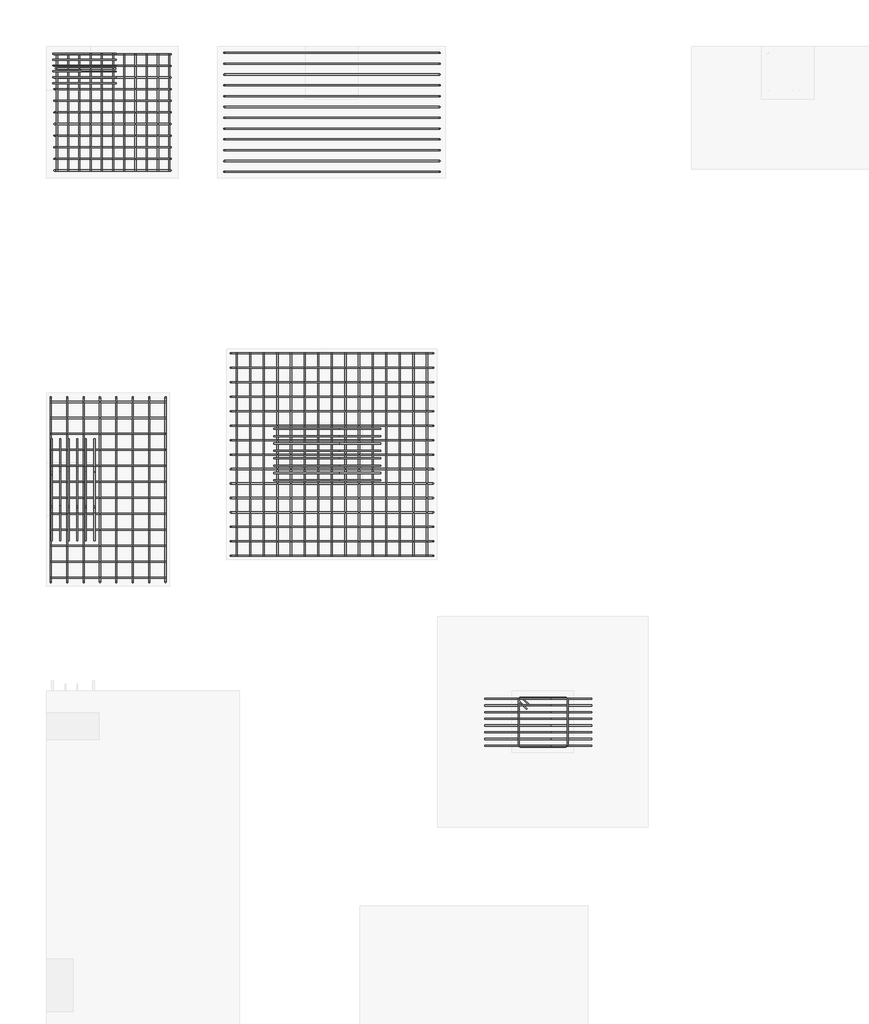
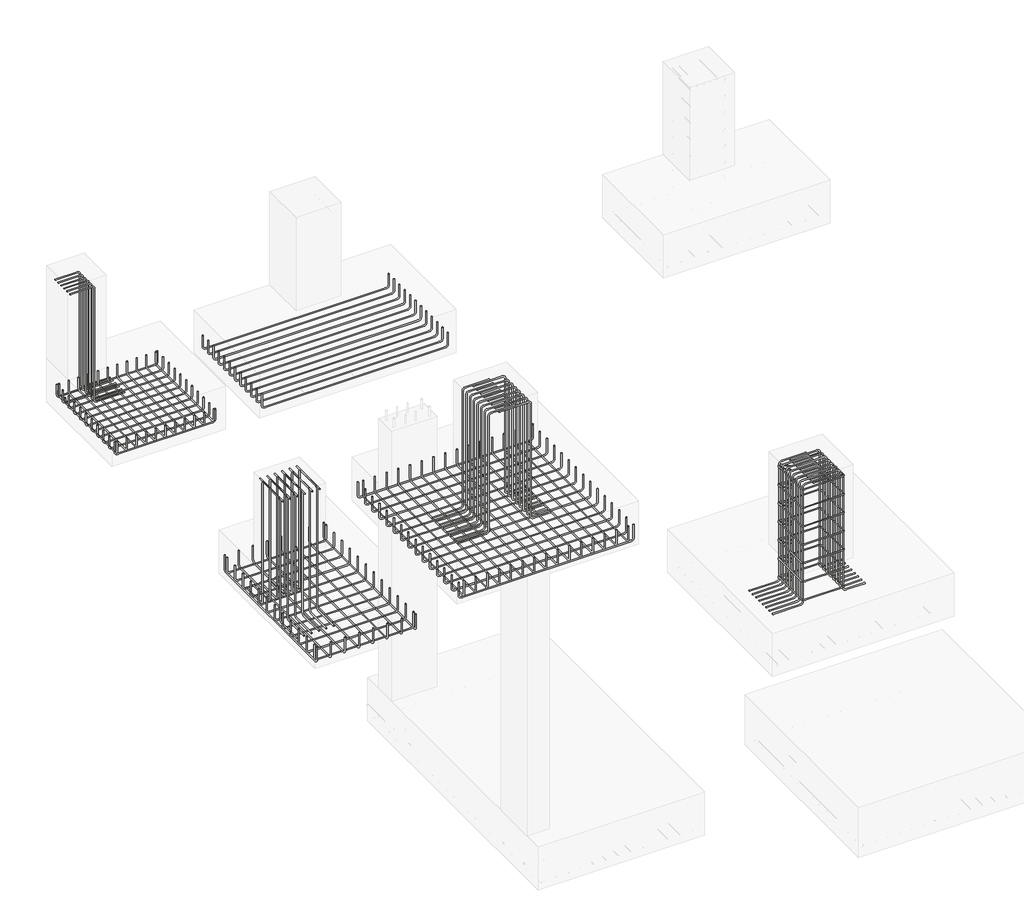
# One storey, part 5 of 6: 16 reinforcing bars.
"""IFC4 building model written with IfcOpenShell, lengths in millimetres."""

from ifc_helpers import new_model, si_unit, point, frame, origin, place, context, project, spatial, polyline, circle_curve, trimmed, segment, composite_curve, source, transform, mapped, element, save
from ifc_brep_helpers import swept_disk

model = new_model("IFC4")

# Units and contexts
model_context = context("Model", 3, world=origin())
ifc_project = project(units=[si_unit("LENGTHUNIT", "METRE", prefix="MILLI")], contexts=[model_context])

# Site, building, storey
site = spatial("IfcSite", under=ifc_project)
building = spatial("IfcBuilding", under=site)
storey = spatial("IfcBuildingStorey", under=building, Elevation=0.0)

# Reinforcing bars
placement = place(None, origin())
reinforcing_bar_shape = source(origin(), model_context, "Body", "SolidModel", [
    swept_disk(composite_curve([segment(polyline([(150341.4232069, -91655.7007776, -254.8), (150341.4232069, -91655.7007776, -365.2)]), True, "CONTINUOUS"), segment(trimmed(circle_curve(frame((150366.4232069, -91655.7007776, -365.2), z_axis=(0.0, -1.0, 0.0), x_axis=(-25.0, 0.0, 0.0)), 25.0), [point((150341.4232069, -91655.7007776, -365.2))], [point((150366.4232069, -91655.7007776, -390.2))], True, "CARTESIAN"), True, "CONTINUOUS"), segment(polyline([(150366.4232069, -91655.7007776, -390.2), (151325.4232069, -91655.7007776, -390.2)]), True, "CONTINUOUS"), segment(trimmed(circle_curve(frame((151325.4232069, -91655.7007776, -365.2), z_axis=(0.0, -1.0, 0.0), x_axis=(0.0, 0.0, -25.0)), 25.0), [point((151325.4232069, -91655.7007776, -390.2))], [point((151350.4232069, -91655.7007776, -365.2))], True, "CARTESIAN"), True, "CONTINUOUS"), segment(polyline([(151350.4232069, -91655.7007776, -365.2), (151350.4232069, -91655.7007776, -254.8)]), True, "CONTINUOUS")], self_intersect=False), 5.0),
])
element("IfcReinforcingBar", 1, at=placement, inside=storey, context=model_context, shape_type="MappedRepresentation", body=[
    mapped(reinforcing_bar_shape, transform((0.0, 0.0, 0.0), x_axis=(1.0, 0.0, 0.0), y_axis=(0.0, 1.0, 0.0), z_axis=(0.0, 0.0, 1.0))),
    mapped(reinforcing_bar_shape, transform((0.0, -100.9, 0.0), x_axis=(1.0, 0.0, 0.0), y_axis=(0.0, 1.0, 0.0), z_axis=(0.0, 0.0, 1.0))),
    mapped(reinforcing_bar_shape, transform((0.0, -201.8, 0.0), x_axis=(1.0, 0.0, 0.0), y_axis=(0.0, 1.0, 0.0), z_axis=(0.0, 0.0, 1.0))),
    mapped(reinforcing_bar_shape, transform((0.0, -302.7, 0.0), x_axis=(1.0, 0.0, 0.0), y_axis=(0.0, 1.0, 0.0), z_axis=(0.0, 0.0, 1.0))),
    mapped(reinforcing_bar_shape, transform((0.0, -403.6, 0.0), x_axis=(1.0, 0.0, 0.0), y_axis=(0.0, 1.0, 0.0), z_axis=(0.0, 0.0, 1.0))),
    mapped(reinforcing_bar_shape, transform((0.0, -504.5, 0.0), x_axis=(1.0, 0.0, 0.0), y_axis=(0.0, 1.0, 0.0), z_axis=(0.0, 0.0, 1.0))),
    mapped(reinforcing_bar_shape, transform((0.0, -605.4, 0.0), x_axis=(1.0, 0.0, 0.0), y_axis=(0.0, 1.0, 0.0), z_axis=(0.0, 0.0, 1.0))),
    mapped(reinforcing_bar_shape, transform((0.0, -706.3, 0.0), x_axis=(1.0, 0.0, 0.0), y_axis=(0.0, 1.0, 0.0), z_axis=(0.0, 0.0, 1.0))),
    mapped(reinforcing_bar_shape, transform((0.0, -807.2, 0.0), x_axis=(1.0, 0.0, 0.0), y_axis=(0.0, 1.0, 0.0), z_axis=(0.0, 0.0, 1.0))),
    mapped(reinforcing_bar_shape, transform((0.0, -908.1, 0.0), x_axis=(1.0, 0.0, 0.0), y_axis=(0.0, 1.0, 0.0), z_axis=(0.0, 0.0, 1.0))),
    mapped(reinforcing_bar_shape, transform((0.0, -1009.0, 0.0), x_axis=(1.0, 0.0, 0.0), y_axis=(0.0, 1.0, 0.0), z_axis=(0.0, 0.0, 1.0))),
])
reinforcing_bar_2_shape = source(origin(), model_context, "Body", "SolidModel", [
    swept_disk(composite_curve([segment(polyline([(150363.1312133, -92664.7007776, -254.8), (150363.1312133, -92664.7007776, -365.2)]), True, "CONTINUOUS"), segment(trimmed(circle_curve(frame((150363.1312133, -92639.7007776, -365.2), z_axis=(1.0, 0.0, 0.0), x_axis=(0.0, -25.0, 0.0)), 25.0), [point((150363.1312133, -92664.7007776, -365.2))], [point((150363.1312133, -92639.7007776, -390.2))], True, "CARTESIAN"), True, "CONTINUOUS"), segment(polyline([(150363.1312133, -92639.7007776, -390.2), (150363.1312133, -91680.7007776, -390.2)]), True, "CONTINUOUS"), segment(trimmed(circle_curve(frame((150363.1312133, -91680.7007776, -365.2), z_axis=(1.0, 0.0, 0.0), x_axis=(0.0, 0.0, -25.0)), 25.0), [point((150363.1312133, -91680.7007776, -390.2))], [point((150363.1312133, -91655.7007776, -365.2))], True, "CARTESIAN"), True, "CONTINUOUS"), segment(polyline([(150363.1312133, -91655.7007776, -365.2), (150363.1312133, -91655.7007776, -254.8)]), True, "CONTINUOUS")], self_intersect=False), 5.0),
])
element("IfcReinforcingBar", 2, at=placement, inside=storey, context=model_context, shape_type="MappedRepresentation", body=[
    mapped(reinforcing_bar_2_shape, transform((0.0, 0.0, 0.0), x_axis=(1.0, 0.0, 0.0), y_axis=(0.0, 1.0, 0.0), z_axis=(0.0, 0.0, 1.0))),
    mapped(reinforcing_bar_2_shape, transform((97.5104958, 0.0, 0.0), x_axis=(1.0, 0.0, 0.0), y_axis=(0.0, 1.0, 0.0), z_axis=(0.0, 0.0, 1.0))),
    mapped(reinforcing_bar_2_shape, transform((195.0209915, 0.0, 0.0), x_axis=(1.0, 0.0, 0.0), y_axis=(0.0, 1.0, 0.0), z_axis=(0.0, 0.0, 1.0))),
    mapped(reinforcing_bar_2_shape, transform((292.5314873, 0.0, 0.0), x_axis=(1.0, 0.0, 0.0), y_axis=(0.0, 1.0, 0.0), z_axis=(0.0, 0.0, 1.0))),
    mapped(reinforcing_bar_2_shape, transform((390.0419831, 0.0, 0.0), x_axis=(1.0, 0.0, 0.0), y_axis=(0.0, 1.0, 0.0), z_axis=(0.0, 0.0, 1.0))),
    mapped(reinforcing_bar_2_shape, transform((487.5524789, 0.0, 0.0), x_axis=(1.0, 0.0, 0.0), y_axis=(0.0, 1.0, 0.0), z_axis=(0.0, 0.0, 1.0))),
    mapped(reinforcing_bar_2_shape, transform((585.0629746, 0.0, 0.0), x_axis=(1.0, 0.0, 0.0), y_axis=(0.0, 1.0, 0.0), z_axis=(0.0, 0.0, 1.0))),
    mapped(reinforcing_bar_2_shape, transform((682.5734704, 0.0, 0.0), x_axis=(1.0, 0.0, 0.0), y_axis=(0.0, 1.0, 0.0), z_axis=(0.0, 0.0, 1.0))),
    mapped(reinforcing_bar_2_shape, transform((780.0839662, 0.0, 0.0), x_axis=(1.0, 0.0, 0.0), y_axis=(0.0, 1.0, 0.0), z_axis=(0.0, 0.0, 1.0))),
    mapped(reinforcing_bar_2_shape, transform((877.5944619, 0.0, 0.0), x_axis=(1.0, 0.0, 0.0), y_axis=(0.0, 1.0, 0.0), z_axis=(0.0, 0.0, 1.0))),
    mapped(reinforcing_bar_2_shape, transform((975.1049577, 0.0, 0.0), x_axis=(1.0, 0.0, 0.0), y_axis=(0.0, 1.0, 0.0), z_axis=(0.0, 0.0, 1.0))),
])
reinforcing_bar_3_shape = source(origin(), model_context, "Body", "SolidModel", [
    swept_disk(composite_curve([segment(polyline([(151306.2232069, -94633.6007776, -254.8), (151306.2232069, -94633.6007776, -397.2)]), True, "CONTINUOUS"), segment(trimmed(circle_curve(frame((151306.2232069, -94658.6007776, -397.2), z_axis=(-1.0, 0.0, 0.0), x_axis=(0.0, 25.0, 0.0)), 25.0), [point((151306.2232069, -94633.6007776, -397.2))], [point((151306.2232069, -94658.6007776, -422.2))], True, "CARTESIAN"), True, "CONTINUOUS"), segment(polyline([(151306.2232069, -94658.6007776, -422.2), (151306.2232069, -96215.0007776, -422.2)]), True, "CONTINUOUS"), segment(trimmed(circle_curve(frame((151306.2232069, -96215.0007776, -397.2), z_axis=(-1.0, 0.0, 0.0), x_axis=(0.0, 0.0, -25.0)), 25.0), [point((151306.2232069, -96215.0007776, -422.2))], [point((151306.2232069, -96240.0007776, -397.2))], True, "CARTESIAN"), True, "CONTINUOUS"), segment(polyline([(151306.2232069, -96240.0007776, -397.2), (151306.2232069, -96240.0007776, -254.8)]), True, "CONTINUOUS")], self_intersect=False), 5.0),
])
element("IfcReinforcingBar", 3, at=placement, inside=storey, context=model_context, shape_type="MappedRepresentation", body=[
    mapped(reinforcing_bar_3_shape, transform((0.0, 0.0, 0.0), x_axis=(1.0, 0.0, 0.0), y_axis=(0.0, 1.0, 0.0), z_axis=(0.0, 0.0, 1.0))),
    mapped(reinforcing_bar_3_shape, transform((-142.4, 0.0, 0.0), x_axis=(1.0, 0.0, 0.0), y_axis=(0.0, 1.0, 0.0), z_axis=(0.0, 0.0, 1.0))),
    mapped(reinforcing_bar_3_shape, transform((-284.8, 0.0, 0.0), x_axis=(1.0, 0.0, 0.0), y_axis=(0.0, 1.0, 0.0), z_axis=(0.0, 0.0, 1.0))),
    mapped(reinforcing_bar_3_shape, transform((-427.2, 0.0, 0.0), x_axis=(1.0, 0.0, 0.0), y_axis=(0.0, 1.0, 0.0), z_axis=(0.0, 0.0, 1.0))),
    mapped(reinforcing_bar_3_shape, transform((-569.6, 0.0, 0.0), x_axis=(1.0, 0.0, 0.0), y_axis=(0.0, 1.0, 0.0), z_axis=(0.0, 0.0, 1.0))),
    mapped(reinforcing_bar_3_shape, transform((-712.0, 0.0, 0.0), x_axis=(1.0, 0.0, 0.0), y_axis=(0.0, 1.0, 0.0), z_axis=(0.0, 0.0, 1.0))),
    mapped(reinforcing_bar_3_shape, transform((-854.4, 0.0, 0.0), x_axis=(1.0, 0.0, 0.0), y_axis=(0.0, 1.0, 0.0), z_axis=(0.0, 0.0, 1.0))),
    mapped(reinforcing_bar_3_shape, transform((-996.8, 0.0, 0.0), x_axis=(1.0, 0.0, 0.0), y_axis=(0.0, 1.0, 0.0), z_axis=(0.0, 0.0, 1.0))),
])
reinforcing_bar_4_shape = source(origin(), model_context, "Body", "SolidModel", [
    swept_disk(composite_curve([segment(polyline([(150309.4232069, -94675.0274486, -254.8), (150309.4232069, -94675.0274486, -397.2)]), True, "CONTINUOUS"), segment(trimmed(circle_curve(frame((150334.4232069, -94675.0274486, -397.2), z_axis=(0.0, -1.0, 0.0), x_axis=(-25.0, 0.0, 0.0)), 25.0), [point((150309.4232069, -94675.0274486, -397.2))], [point((150334.4232069, -94675.0274486, -422.2))], True, "CARTESIAN"), True, "CONTINUOUS"), segment(polyline([(150334.4232069, -94675.0274486, -422.2), (151281.2232069, -94675.0274486, -422.2)]), True, "CONTINUOUS"), segment(trimmed(circle_curve(frame((151281.2232069, -94675.0274486, -397.2), z_axis=(0.0, -1.0, 0.0), x_axis=(0.0, 0.0, -25.0)), 25.0), [point((151281.2232069, -94675.0274486, -422.2))], [point((151306.2232069, -94675.0274486, -397.2))], True, "CARTESIAN"), True, "CONTINUOUS"), segment(polyline([(151306.2232069, -94675.0274486, -397.2), (151306.2232069, -94675.0274486, -254.8)]), True, "CONTINUOUS")], self_intersect=False), 5.0),
])
element("IfcReinforcingBar", 4, at=placement, inside=storey, context=model_context, shape_type="MappedRepresentation", body=[
    mapped(reinforcing_bar_4_shape, transform((0.0, 0.0, 0.0), x_axis=(1.0, 0.0, 0.0), y_axis=(0.0, 1.0, 0.0), z_axis=(0.0, 0.0, 1.0))),
    mapped(reinforcing_bar_4_shape, transform((0.0, -138.7698059, 0.0), x_axis=(1.0, 0.0, 0.0), y_axis=(0.0, 1.0, 0.0), z_axis=(0.0, 0.0, 1.0))),
    mapped(reinforcing_bar_4_shape, transform((0.0, -277.5396119, 0.0), x_axis=(1.0, 0.0, 0.0), y_axis=(0.0, 1.0, 0.0), z_axis=(0.0, 0.0, 1.0))),
    mapped(reinforcing_bar_4_shape, transform((0.0, -416.3094178, 0.0), x_axis=(1.0, 0.0, 0.0), y_axis=(0.0, 1.0, 0.0), z_axis=(0.0, 0.0, 1.0))),
    mapped(reinforcing_bar_4_shape, transform((0.0, -555.0792237, 0.0), x_axis=(1.0, 0.0, 0.0), y_axis=(0.0, 1.0, 0.0), z_axis=(0.0, 0.0, 1.0))),
    mapped(reinforcing_bar_4_shape, transform((0.0, -693.8490296, 0.0), x_axis=(1.0, 0.0, 0.0), y_axis=(0.0, 1.0, 0.0), z_axis=(0.0, 0.0, 1.0))),
    mapped(reinforcing_bar_4_shape, transform((0.0, -832.6188356, 0.0), x_axis=(1.0, 0.0, 0.0), y_axis=(0.0, 1.0, 0.0), z_axis=(0.0, 0.0, 1.0))),
    mapped(reinforcing_bar_4_shape, transform((0.0, -971.3886415, 0.0), x_axis=(1.0, 0.0, 0.0), y_axis=(0.0, 1.0, 0.0), z_axis=(0.0, 0.0, 1.0))),
    mapped(reinforcing_bar_4_shape, transform((0.0, -1110.1584474, 0.0), x_axis=(1.0, 0.0, 0.0), y_axis=(0.0, 1.0, 0.0), z_axis=(0.0, 0.0, 1.0))),
    mapped(reinforcing_bar_4_shape, transform((0.0, -1248.9282533, 0.0), x_axis=(1.0, 0.0, 0.0), y_axis=(0.0, 1.0, 0.0), z_axis=(0.0, 0.0, 1.0))),
    mapped(reinforcing_bar_4_shape, transform((0.0, -1387.6980593, 0.0), x_axis=(1.0, 0.0, 0.0), y_axis=(0.0, 1.0, 0.0), z_axis=(0.0, 0.0, 1.0))),
    mapped(reinforcing_bar_4_shape, transform((0.0, -1526.4678652, 0.0), x_axis=(1.0, 0.0, 0.0), y_axis=(0.0, 1.0, 0.0), z_axis=(0.0, 0.0, 1.0))),
])
reinforcing_bar_5_shape = source(origin(), model_context, "Body", "SolidModel", [
    swept_disk(composite_curve([segment(polyline([(151815.3232069, -91643.7007776, -254.8), (151815.3232069, -91643.7007776, -377.2)]), True, "CONTINUOUS"), segment(trimmed(circle_curve(frame((151840.3232069, -91643.7007776, -377.2), z_axis=(0.0, -1.0, 0.0), x_axis=(-25.0, 0.0, 0.0)), 25.0), [point((151815.3232069, -91643.7007776, -377.2))], [point((151840.3232069, -91643.7007776, -402.2))], True, "CARTESIAN"), True, "CONTINUOUS"), segment(polyline([(151840.3232069, -91643.7007776, -402.2), (153661.5232069, -91643.7007776, -402.2)]), True, "CONTINUOUS"), segment(trimmed(circle_curve(frame((153661.5232069, -91643.7007776, -377.2), z_axis=(0.0, -1.0, 0.0), x_axis=(0.0, 0.0, -25.0)), 25.0), [point((153661.5232069, -91643.7007776, -402.2))], [point((153686.5232069, -91643.7007776, -377.2))], True, "CARTESIAN"), True, "CONTINUOUS"), segment(polyline([(153686.5232069, -91643.7007776, -377.2), (153686.5232069, -91643.7007776, -254.8)]), True, "CONTINUOUS")], self_intersect=False), 5.0),
])
element("IfcReinforcingBar", 5, at=placement, inside=storey, context=model_context, shape_type="MappedRepresentation", body=[
    mapped(reinforcing_bar_5_shape, transform((0.0, 0.0, 0.0), x_axis=(1.0, 0.0, 0.0), y_axis=(0.0, 1.0, 0.0), z_axis=(0.0, 0.0, 1.0))),
    mapped(reinforcing_bar_5_shape, transform((0.0, -93.9090909, 0.0), x_axis=(1.0, 0.0, 0.0), y_axis=(0.0, 1.0, 0.0), z_axis=(0.0, 0.0, 1.0))),
    mapped(reinforcing_bar_5_shape, transform((0.0, -187.8181818, 0.0), x_axis=(1.0, 0.0, 0.0), y_axis=(0.0, 1.0, 0.0), z_axis=(0.0, 0.0, 1.0))),
    mapped(reinforcing_bar_5_shape, transform((0.0, -281.7272727, 0.0), x_axis=(1.0, 0.0, 0.0), y_axis=(0.0, 1.0, 0.0), z_axis=(0.0, 0.0, 1.0))),
    mapped(reinforcing_bar_5_shape, transform((0.0, -375.6363636, 0.0), x_axis=(1.0, 0.0, 0.0), y_axis=(0.0, 1.0, 0.0), z_axis=(0.0, 0.0, 1.0))),
    mapped(reinforcing_bar_5_shape, transform((0.0, -469.5454545, 0.0), x_axis=(1.0, 0.0, 0.0), y_axis=(0.0, 1.0, 0.0), z_axis=(0.0, 0.0, 1.0))),
    mapped(reinforcing_bar_5_shape, transform((0.0, -563.4545455, 0.0), x_axis=(1.0, 0.0, 0.0), y_axis=(0.0, 1.0, 0.0), z_axis=(0.0, 0.0, 1.0))),
    mapped(reinforcing_bar_5_shape, transform((0.0, -657.3636364, 0.0), x_axis=(1.0, 0.0, 0.0), y_axis=(0.0, 1.0, 0.0), z_axis=(0.0, 0.0, 1.0))),
    mapped(reinforcing_bar_5_shape, transform((0.0, -751.2727273, 0.0), x_axis=(1.0, 0.0, 0.0), y_axis=(0.0, 1.0, 0.0), z_axis=(0.0, 0.0, 1.0))),
    mapped(reinforcing_bar_5_shape, transform((0.0, -845.1818182, 0.0), x_axis=(1.0, 0.0, 0.0), y_axis=(0.0, 1.0, 0.0), z_axis=(0.0, 0.0, 1.0))),
    mapped(reinforcing_bar_5_shape, transform((0.0, -939.0909091, 0.0), x_axis=(1.0, 0.0, 0.0), y_axis=(0.0, 1.0, 0.0), z_axis=(0.0, 0.0, 1.0))),
    mapped(reinforcing_bar_5_shape, transform((0.0, -1033.0, 0.0), x_axis=(1.0, 0.0, 0.0), y_axis=(0.0, 1.0, 0.0), z_axis=(0.0, 0.0, 1.0))),
])
reinforcing_bar_6_shape = source(origin(), model_context, "Body", "SolidModel", [
    swept_disk(composite_curve([segment(polyline([(151871.5232069, -94252.6007776, -254.8), (151871.5232069, -94252.6007776, -397.2)]), True, "CONTINUOUS"), segment(trimmed(circle_curve(frame((151896.5232069, -94252.6007776, -397.2), z_axis=(0.0, -1.0, 0.0), x_axis=(-25.0, 0.0, 0.0)), 25.0), [point((151871.5232069, -94252.6007776, -397.2))], [point((151896.5232069, -94252.6007776, -422.2))], True, "CARTESIAN"), True, "CONTINUOUS"), segment(polyline([(151896.5232069, -94252.6007776, -422.2), (153605.3232069, -94252.6007776, -422.2)]), True, "CONTINUOUS"), segment(trimmed(circle_curve(frame((153605.3232069, -94252.6007776, -397.2), z_axis=(0.0, -1.0, 0.0), x_axis=(0.0, 0.0, -25.0)), 25.0), [point((153605.3232069, -94252.6007776, -422.2))], [point((153630.3232069, -94252.6007776, -397.2))], True, "CARTESIAN"), True, "CONTINUOUS"), segment(polyline([(153630.3232069, -94252.6007776, -397.2), (153630.3232069, -94252.6007776, -254.8)]), True, "CONTINUOUS")], self_intersect=False), 5.0),
])
element("IfcReinforcingBar", 6, at=placement, inside=storey, context=model_context, shape_type="MappedRepresentation", body=[
    mapped(reinforcing_bar_6_shape, transform((0.0, 0.0, 0.0), x_axis=(1.0, 0.0, 0.0), y_axis=(0.0, 1.0, 0.0), z_axis=(0.0, 0.0, 1.0))),
    mapped(reinforcing_bar_6_shape, transform((0.0, -125.6285714, 0.0), x_axis=(1.0, 0.0, 0.0), y_axis=(0.0, 1.0, 0.0), z_axis=(0.0, 0.0, 1.0))),
    mapped(reinforcing_bar_6_shape, transform((0.0, -251.2571429, 0.0), x_axis=(1.0, 0.0, 0.0), y_axis=(0.0, 1.0, 0.0), z_axis=(0.0, 0.0, 1.0))),
    mapped(reinforcing_bar_6_shape, transform((0.0, -376.8857143, 0.0), x_axis=(1.0, 0.0, 0.0), y_axis=(0.0, 1.0, 0.0), z_axis=(0.0, 0.0, 1.0))),
    mapped(reinforcing_bar_6_shape, transform((0.0, -502.5142857, 0.0), x_axis=(1.0, 0.0, 0.0), y_axis=(0.0, 1.0, 0.0), z_axis=(0.0, 0.0, 1.0))),
    mapped(reinforcing_bar_6_shape, transform((0.0, -628.1428571, 0.0), x_axis=(1.0, 0.0, 0.0), y_axis=(0.0, 1.0, 0.0), z_axis=(0.0, 0.0, 1.0))),
    mapped(reinforcing_bar_6_shape, transform((0.0, -753.7714286, 0.0), x_axis=(1.0, 0.0, 0.0), y_axis=(0.0, 1.0, 0.0), z_axis=(0.0, 0.0, 1.0))),
    mapped(reinforcing_bar_6_shape, transform((0.0, -879.4, 0.0), x_axis=(1.0, 0.0, 0.0), y_axis=(0.0, 1.0, 0.0), z_axis=(0.0, 0.0, 1.0))),
    mapped(reinforcing_bar_6_shape, transform((0.0, -1005.0285714, 0.0), x_axis=(1.0, 0.0, 0.0), y_axis=(0.0, 1.0, 0.0), z_axis=(0.0, 0.0, 1.0))),
    mapped(reinforcing_bar_6_shape, transform((0.0, -1130.6571429, 0.0), x_axis=(1.0, 0.0, 0.0), y_axis=(0.0, 1.0, 0.0), z_axis=(0.0, 0.0, 1.0))),
    mapped(reinforcing_bar_6_shape, transform((0.0, -1256.2857143, 0.0), x_axis=(1.0, 0.0, 0.0), y_axis=(0.0, 1.0, 0.0), z_axis=(0.0, 0.0, 1.0))),
    mapped(reinforcing_bar_6_shape, transform((0.0, -1381.9142857, 0.0), x_axis=(1.0, 0.0, 0.0), y_axis=(0.0, 1.0, 0.0), z_axis=(0.0, 0.0, 1.0))),
    mapped(reinforcing_bar_6_shape, transform((0.0, -1507.5428571, 0.0), x_axis=(1.0, 0.0, 0.0), y_axis=(0.0, 1.0, 0.0), z_axis=(0.0, 0.0, 1.0))),
    mapped(reinforcing_bar_6_shape, transform((0.0, -1633.1714286, 0.0), x_axis=(1.0, 0.0, 0.0), y_axis=(0.0, 1.0, 0.0), z_axis=(0.0, 0.0, 1.0))),
    mapped(reinforcing_bar_6_shape, transform((0.0, -1758.8, 0.0), x_axis=(1.0, 0.0, 0.0), y_axis=(0.0, 1.0, 0.0), z_axis=(0.0, 0.0, 1.0))),
])
reinforcing_bar_7_shape = source(origin(), model_context, "Body", "SolidModel", [
    swept_disk(composite_curve([segment(polyline([(151923.5391163, -96011.4007776, -254.8), (151923.5391163, -96011.4007776, -397.2)]), True, "CONTINUOUS"), segment(trimmed(circle_curve(frame((151923.5391163, -95986.4007776, -397.2), z_axis=(1.0, 0.0, 0.0), x_axis=(0.0, -25.0, 0.0)), 25.0), [point((151923.5391163, -96011.4007776, -397.2))], [point((151923.5391163, -95986.4007776, -422.2))], True, "CARTESIAN"), True, "CONTINUOUS"), segment(polyline([(151923.5391163, -95986.4007776, -422.2), (151923.5391163, -94277.6007776, -422.2)]), True, "CONTINUOUS"), segment(trimmed(circle_curve(frame((151923.5391163, -94277.6007776, -397.2), z_axis=(1.0, 0.0, 0.0), x_axis=(0.0, 0.0, -25.0)), 25.0), [point((151923.5391163, -94277.6007776, -422.2))], [point((151923.5391163, -94252.6007776, -397.2))], True, "CARTESIAN"), True, "CONTINUOUS"), segment(polyline([(151923.5391163, -94252.6007776, -397.2), (151923.5391163, -94252.6007776, -254.8)]), True, "CONTINUOUS")], self_intersect=False), 5.0),
])
element("IfcReinforcingBar", 7, at=placement, inside=storey, context=model_context, shape_type="MappedRepresentation", body=[
    mapped(reinforcing_bar_7_shape, transform((0.0, 0.0, 0.0), x_axis=(1.0, 0.0, 0.0), y_axis=(0.0, 1.0, 0.0), z_axis=(0.0, 0.0, 1.0))),
    mapped(reinforcing_bar_7_shape, transform((118.1173845, 0.0, 0.0), x_axis=(1.0, 0.0, 0.0), y_axis=(0.0, 1.0, 0.0), z_axis=(0.0, 0.0, 1.0))),
    mapped(reinforcing_bar_7_shape, transform((236.2347691, 0.0, 0.0), x_axis=(1.0, 0.0, 0.0), y_axis=(0.0, 1.0, 0.0), z_axis=(0.0, 0.0, 1.0))),
    mapped(reinforcing_bar_7_shape, transform((354.3521536, 0.0, 0.0), x_axis=(1.0, 0.0, 0.0), y_axis=(0.0, 1.0, 0.0), z_axis=(0.0, 0.0, 1.0))),
    mapped(reinforcing_bar_7_shape, transform((472.4695381, 0.0, 0.0), x_axis=(1.0, 0.0, 0.0), y_axis=(0.0, 1.0, 0.0), z_axis=(0.0, 0.0, 1.0))),
    mapped(reinforcing_bar_7_shape, transform((590.5869227, 0.0, 0.0), x_axis=(1.0, 0.0, 0.0), y_axis=(0.0, 1.0, 0.0), z_axis=(0.0, 0.0, 1.0))),
    mapped(reinforcing_bar_7_shape, transform((708.7043072, 0.0, 0.0), x_axis=(1.0, 0.0, 0.0), y_axis=(0.0, 1.0, 0.0), z_axis=(0.0, 0.0, 1.0))),
    mapped(reinforcing_bar_7_shape, transform((826.8216917, 0.0, 0.0), x_axis=(1.0, 0.0, 0.0), y_axis=(0.0, 1.0, 0.0), z_axis=(0.0, 0.0, 1.0))),
    mapped(reinforcing_bar_7_shape, transform((944.9390763, 0.0, 0.0), x_axis=(1.0, 0.0, 0.0), y_axis=(0.0, 1.0, 0.0), z_axis=(0.0, 0.0, 1.0))),
    mapped(reinforcing_bar_7_shape, transform((1063.0564608, 0.0, 0.0), x_axis=(1.0, 0.0, 0.0), y_axis=(0.0, 1.0, 0.0), z_axis=(0.0, 0.0, 1.0))),
    mapped(reinforcing_bar_7_shape, transform((1181.1738453, 0.0, 0.0), x_axis=(1.0, 0.0, 0.0), y_axis=(0.0, 1.0, 0.0), z_axis=(0.0, 0.0, 1.0))),
    mapped(reinforcing_bar_7_shape, transform((1299.2912299, 0.0, 0.0), x_axis=(1.0, 0.0, 0.0), y_axis=(0.0, 1.0, 0.0), z_axis=(0.0, 0.0, 1.0))),
    mapped(reinforcing_bar_7_shape, transform((1417.4086144, 0.0, 0.0), x_axis=(1.0, 0.0, 0.0), y_axis=(0.0, 1.0, 0.0), z_axis=(0.0, 0.0, 1.0))),
    mapped(reinforcing_bar_7_shape, transform((1535.5259989, 0.0, 0.0), x_axis=(1.0, 0.0, 0.0), y_axis=(0.0, 1.0, 0.0), z_axis=(0.0, 0.0, 1.0))),
    mapped(reinforcing_bar_7_shape, transform((1653.6433835, 0.0, 0.0), x_axis=(1.0, 0.0, 0.0), y_axis=(0.0, 1.0, 0.0), z_axis=(0.0, 0.0, 1.0))),
])
reinforcing_bar_8_shape = source(origin(), model_context, "Body", "SolidModel", [
    swept_disk(composite_curve([segment(polyline([(150324.4232069, -91907.7007776, 863.1556942), (150552.0732069, -91907.7007776, 863.1556942)]), True, "CONTINUOUS"), segment(trimmed(circle_curve(frame((150552.0732069, -91907.7007776, 843.1556942), z_axis=(0.0, 1.0, 0.0), x_axis=(0.0, 0.0, 20.0)), 20.0), [point((150552.0732069, -91907.7007776, 863.1556942))], [point((150572.0732069, -91907.7007776, 843.1556942))], True, "CARTESIAN"), True, "CONTINUOUS"), segment(polyline([(150572.0732069, -91907.7007776, 843.1556942), (150572.0732069, -91907.7007776, -350.9334646)]), True, "CONTINUOUS"), segment(trimmed(circle_curve(frame((150592.0732069, -91907.7007776, -350.9334646), z_axis=(0.0, -1.0, 0.0), x_axis=(-20.0, 0.0, 0.0)), 20.0), [point((150572.0732069, -91907.7007776, -350.9334646))], [point((150592.0732069, -91907.7007776, -370.9334646))], True, "CARTESIAN"), True, "CONTINUOUS"), segment(polyline([(150592.0732069, -91907.7007776, -370.9334646), (150876.8732069, -91907.7007776, -370.9334646)]), True, "CONTINUOUS")], self_intersect=False), 4.0),
])
element("IfcReinforcingBar", 8, at=placement, inside=storey, context=model_context, shape_type="MappedRepresentation", body=[
    mapped(reinforcing_bar_8_shape, transform((0.0, 0.0, 0.0), x_axis=(1.0, 0.0, 0.0), y_axis=(0.0, 1.0, 0.0), z_axis=(0.0, 0.0, 1.0))),
    mapped(reinforcing_bar_8_shape, transform((0.0, 51.4, 0.0), x_axis=(1.0, 0.0, 0.0), y_axis=(0.0, 1.0, 0.0), z_axis=(0.0, 0.0, 1.0))),
    mapped(reinforcing_bar_8_shape, transform((0.0, 102.8, 0.0), x_axis=(1.0, 0.0, 0.0), y_axis=(0.0, 1.0, 0.0), z_axis=(0.0, 0.0, 1.0))),
    mapped(reinforcing_bar_8_shape, transform((0.0, 154.2, 0.0), x_axis=(1.0, 0.0, 0.0), y_axis=(0.0, 1.0, 0.0), z_axis=(0.0, 0.0, 1.0))),
    mapped(reinforcing_bar_8_shape, transform((0.0, 205.6, 0.0), x_axis=(1.0, 0.0, 0.0), y_axis=(0.0, 1.0, 0.0), z_axis=(0.0, 0.0, 1.0))),
    mapped(reinforcing_bar_8_shape, transform((0.0, 257.0, 0.0), x_axis=(1.0, 0.0, 0.0), y_axis=(0.0, 1.0, 0.0), z_axis=(0.0, 0.0, 1.0))),
])
reinforcing_bar_9_shape = source(origin(), model_context, "Body", "SolidModel", [
    swept_disk(composite_curve([segment(polyline([(150871.5772931, -91779.2007776, -387.2757427), (150376.7835327, -91779.2007776, -387.2757427)]), True, "CONTINUOUS"), segment(trimmed(circle_curve(frame((150376.7835327, -91779.2007776, -362.2757427), z_axis=(0.0, 1.0, 0.0), x_axis=(0.0, 0.0, -25.0)), 25.0), [point((150376.7835327, -91779.2007776, -387.2757427))], [point((150351.7835327, -91779.2007776, -362.2757427))], True, "CARTESIAN"), True, "CONTINUOUS"), segment(polyline([(150351.7835327, -91779.2007776, -362.2757427), (150351.7835327, -91779.2007776, -324.6265395)]), True, "CONTINUOUS")], self_intersect=False), 5.0),
])
element("IfcReinforcingBar", 9, at=placement, inside=storey, context=model_context, shape_type="MappedRepresentation", body=[
    mapped(reinforcing_bar_9_shape, transform((0.0, 0.0, 0.0), x_axis=(1.0, 0.0, 0.0), y_axis=(0.0, 1.0, 0.0), z_axis=(0.0, 0.0, 1.0))),
    mapped(reinforcing_bar_9_shape, transform((0.0, 123.5, 0.0), x_axis=(1.0, 0.0, 0.0), y_axis=(0.0, 1.0, 0.0), z_axis=(0.0, 0.0, 1.0))),
])
reinforcing_bar_10_shape = source(origin(), model_context, "Body", "SolidModel", [
    swept_disk(composite_curve([segment(polyline([(154649.8526774, -97252.4007776, 904.4108031), (154408.1526774, -97252.4007776, 904.4108031)]), True, "CONTINUOUS"), segment(trimmed(circle_curve(frame((154408.1526774, -97252.4007776, 879.4108031), z_axis=(0.0, -1.0, 0.0), x_axis=(0.0, 0.0, 25.0)), 25.0), [point((154408.1526774, -97252.4007776, 904.4108031))], [point((154383.1526774, -97252.4007776, 879.4108031))], True, "CARTESIAN"), True, "CONTINUOUS"), segment(polyline([(154383.1526774, -97252.4007776, 879.4108031), (154383.1526774, -97252.4007776, -340.5891969)]), True, "CONTINUOUS"), segment(trimmed(circle_curve(frame((154358.1526774, -97252.4007776, -340.5891969), z_axis=(0.0, 1.0, 0.0), x_axis=(25.0, 0.0, 0.0)), 25.0), [point((154383.1526774, -97252.4007776, -340.5891969))], [point((154358.1526774, -97252.4007776, -365.5891969))], True, "CARTESIAN"), True, "CONTINUOUS"), segment(polyline([(154358.1526774, -97252.4007776, -365.5891969), (154078.3526774, -97252.4007776, -365.5891969)]), True, "CONTINUOUS")], self_intersect=False), 5.0),
])
element("IfcReinforcingBar", 10, at=placement, inside=storey, context=model_context, shape_type="MappedRepresentation", body=[
    mapped(reinforcing_bar_10_shape, transform((0.0, 0.0, 0.0), x_axis=(1.0, 0.0, 0.0), y_axis=(0.0, 1.0, 0.0), z_axis=(0.0, 0.0, 1.0))),
    mapped(reinforcing_bar_10_shape, transform((0.0, -58.2, 0.0), x_axis=(1.0, 0.0, 0.0), y_axis=(0.0, 1.0, 0.0), z_axis=(0.0, 0.0, 1.0))),
    mapped(reinforcing_bar_10_shape, transform((0.0, -116.4, 0.0), x_axis=(1.0, 0.0, 0.0), y_axis=(0.0, 1.0, 0.0), z_axis=(0.0, 0.0, 1.0))),
    mapped(reinforcing_bar_10_shape, transform((0.0, -174.6, 0.0), x_axis=(1.0, 0.0, 0.0), y_axis=(0.0, 1.0, 0.0), z_axis=(0.0, 0.0, 1.0))),
    mapped(reinforcing_bar_10_shape, transform((0.0, -232.8, 0.0), x_axis=(1.0, 0.0, 0.0), y_axis=(0.0, 1.0, 0.0), z_axis=(0.0, 0.0, 1.0))),
    mapped(reinforcing_bar_10_shape, transform((0.0, -291.0, 0.0), x_axis=(1.0, 0.0, 0.0), y_axis=(0.0, 1.0, 0.0), z_axis=(0.0, 0.0, 1.0))),
    mapped(reinforcing_bar_10_shape, transform((0.0, -349.2, 0.0), x_axis=(1.0, 0.0, 0.0), y_axis=(0.0, 1.0, 0.0), z_axis=(0.0, 0.0, 1.0))),
    mapped(reinforcing_bar_10_shape, transform((0.0, -407.4, 0.0), x_axis=(1.0, 0.0, 0.0), y_axis=(0.0, 1.0, 0.0), z_axis=(0.0, 0.0, 1.0))),
])
reinforcing_bar_11_shape = source(origin(), model_context, "Body", "SolidModel", [
    swept_disk(composite_curve([segment(polyline([(154487.7597873, -97659.8007776, 889.0558214), (154764.1805846, -97659.8007776, 889.0558214)]), True, "CONTINUOUS"), segment(trimmed(circle_curve(frame((154764.1805846, -97659.8007776, 864.0558214), z_axis=(0.0, 1.0, 0.0), x_axis=(0.0, 0.0, 25.0)), 25.0), [point((154764.1805846, -97659.8007776, 889.0558214))], [point((154789.1805846, -97659.8007776, 864.0558214))], True, "CARTESIAN"), True, "CONTINUOUS"), segment(polyline([(154789.1805846, -97659.8007776, 864.0558214), (154789.1805846, -97659.8007776, -336.4777139)]), True, "CONTINUOUS"), segment(trimmed(circle_curve(frame((154814.1805846, -97659.8007776, -336.4777139), z_axis=(0.0, -1.0, 0.0), x_axis=(-25.0, 0.0, 0.0)), 25.0), [point((154789.1805846, -97659.8007776, -336.4777139))], [point((154814.1805846, -97659.8007776, -361.4777139))], True, "CARTESIAN"), True, "CONTINUOUS"), segment(polyline([(154814.1805846, -97659.8007776, -361.4777139), (155008.4597873, -97659.8007776, -361.4777139)]), True, "CONTINUOUS")], self_intersect=False), 5.0),
])
element("IfcReinforcingBar", 11, at=placement, inside=storey, context=model_context, shape_type="MappedRepresentation", body=[
    mapped(reinforcing_bar_11_shape, transform((0.0, 0.0, 0.0), x_axis=(1.0, 0.0, 0.0), y_axis=(0.0, 1.0, 0.0), z_axis=(0.0, 0.0, 1.0))),
    mapped(reinforcing_bar_11_shape, transform((0.0, 58.2, 0.0), x_axis=(1.0, 0.0, 0.0), y_axis=(0.0, 1.0, 0.0), z_axis=(0.0, 0.0, 1.0))),
    mapped(reinforcing_bar_11_shape, transform((0.0, 116.4, 0.0), x_axis=(1.0, 0.0, 0.0), y_axis=(0.0, 1.0, 0.0), z_axis=(0.0, 0.0, 1.0))),
    mapped(reinforcing_bar_11_shape, transform((0.0, 174.6, 0.0), x_axis=(1.0, 0.0, 0.0), y_axis=(0.0, 1.0, 0.0), z_axis=(0.0, 0.0, 1.0))),
    mapped(reinforcing_bar_11_shape, transform((0.0, 232.8, 0.0), x_axis=(1.0, 0.0, 0.0), y_axis=(0.0, 1.0, 0.0), z_axis=(0.0, 0.0, 1.0))),
    mapped(reinforcing_bar_11_shape, transform((0.0, 291.0, 0.0), x_axis=(1.0, 0.0, 0.0), y_axis=(0.0, 1.0, 0.0), z_axis=(0.0, 0.0, 1.0))),
    mapped(reinforcing_bar_11_shape, transform((0.0, 349.2, 0.0), x_axis=(1.0, 0.0, 0.0), y_axis=(0.0, 1.0, 0.0), z_axis=(0.0, 0.0, 1.0))),
    mapped(reinforcing_bar_11_shape, transform((0.0, 407.4, 0.0), x_axis=(1.0, 0.0, 0.0), y_axis=(0.0, 1.0, 0.0), z_axis=(0.0, 0.0, 1.0))),
])
reinforcing_bar_12_shape = source(origin(), model_context, "Body", "SolidModel", [
    swept_disk(composite_curve([segment(polyline([(154471.2694373, -97313.605359, -318.2339629), (154406.9227202, -97249.258642, -318.2339629)]), True, "CONTINUOUS"), segment(trimmed(circle_curve(frame((154392.7805846, -97263.4007776, -318.2339629), z_axis=(0.0, 0.0, 1.0), x_axis=(14.14213560000644, 14.14213560000644, 0.0)), 20.0), [point((154406.9227202, -97249.258642, -318.2339629))], [point((154372.7805846, -97263.4007776, -318.2339629))], True, "CARTESIAN"), True, "CONTINUOUS"), segment(polyline([(154372.7805846, -97263.4007776, -318.2339629), (154372.7805846, -97648.8007776, -318.2339629)]), True, "CONTINUOUS"), segment(trimmed(circle_curve(frame((154392.7805846, -97648.8007776, -318.2339629), z_axis=(0.0, 0.0, 1.0), x_axis=(-20.0, 0.0, 0.0)), 20.0), [point((154372.7805846, -97648.8007776, -318.2339629))], [point((154392.7805846, -97668.8007776, -318.2339629))], True, "CARTESIAN"), True, "CONTINUOUS"), segment(polyline([(154392.7805846, -97668.8007776, -318.2339629), (154778.1805846, -97668.8007776, -318.2339629)]), True, "CONTINUOUS"), segment(trimmed(circle_curve(frame((154778.1805846, -97648.8043132, -318.6100131), z_axis=(0.0, 0.01880250526134292, 0.9998232172718822), x_axis=(0.0, -19.99646439999924, 0.37605020000000877)), 20.0), [point((154778.1805846, -97668.8007776, -318.2339629))], [point((154798.1805846, -97648.8043132, -318.6100131))], True, "CARTESIAN"), True, "CONTINUOUS"), segment(polyline([(154798.1805846, -97648.8043132, -318.6100131), (154798.1805846, -97263.3972419, -325.8579128)]), True, "CONTINUOUS"), segment(trimmed(circle_curve(frame((154778.1805846, -97263.3972419, -325.8579128), z_axis=(0.0, 0.01880250526134292, 0.9998232172718822), x_axis=(20.0, 0.0, 0.0)), 20.0), [point((154798.1805846, -97263.3972419, -325.8579128))], [point((154778.1805846, -97243.4007776, -326.2339629))], True, "CARTESIAN"), True, "CONTINUOUS"), segment(polyline([(154778.1805846, -97243.4007776, -326.2339629), (154392.7805846, -97243.4007776, -326.2339629)]), True, "CONTINUOUS"), segment(trimmed(circle_curve(frame((154392.7805846, -97263.4007776, -326.2339629), z_axis=(0.0, 0.0, 1.0), x_axis=(0.0, 20.0, 0.0)), 20.0), [point((154392.7805846, -97243.4007776, -326.2339629))], [point((154378.638449, -97277.5429132, -326.2339629))], True, "CARTESIAN"), True, "CONTINUOUS"), segment(polyline([(154378.638449, -97277.5429132, -326.2339629), (154442.985166, -97341.8896303, -326.2339629)]), True, "CONTINUOUS")], self_intersect=False), 4.0),
])
element("IfcReinforcingBar", 12, at=placement, inside=storey, context=model_context, shape_type="MappedRepresentation", body=[
    mapped(reinforcing_bar_12_shape, transform((0.0, 0.0, 0.0), x_axis=(1.0, 0.0, 0.0), y_axis=(0.0, 1.0, 0.0), z_axis=(0.0, 0.0, 1.0))),
    mapped(reinforcing_bar_12_shape, transform((0.0, 0.0, 196.2536444), x_axis=(1.0, 0.0, 0.0), y_axis=(0.0, 1.0, 0.0), z_axis=(0.0, 0.0, 1.0))),
    mapped(reinforcing_bar_12_shape, transform((0.0, 0.0, 392.5072887), x_axis=(1.0, 0.0, 0.0), y_axis=(0.0, 1.0, 0.0), z_axis=(0.0, 0.0, 1.0))),
    mapped(reinforcing_bar_12_shape, transform((0.0, 0.0, 588.7609331), x_axis=(1.0, 0.0, 0.0), y_axis=(0.0, 1.0, 0.0), z_axis=(0.0, 0.0, 1.0))),
    mapped(reinforcing_bar_12_shape, transform((0.0, 0.0, 785.0145774), x_axis=(1.0, 0.0, 0.0), y_axis=(0.0, 1.0, 0.0), z_axis=(0.0, 0.0, 1.0))),
    mapped(reinforcing_bar_12_shape, transform((0.0, 0.0, 981.2682218), x_axis=(1.0, 0.0, 0.0), y_axis=(0.0, 1.0, 0.0), z_axis=(0.0, 0.0, 1.0))),
    mapped(reinforcing_bar_12_shape, transform((0.0, 0.0, 1177.5218661), x_axis=(1.0, 0.0, 0.0), y_axis=(0.0, 1.0, 0.0), z_axis=(0.0, 0.0, 1.0))),
])
reinforcing_bar_13_shape = source(origin(), model_context, "Body", "SolidModel", [
    swept_disk(composite_curve([segment(polyline([(152815.2952998, -94908.3007776, 904.4108031), (152573.5952998, -94908.3007776, 904.4108031)]), True, "CONTINUOUS"), segment(trimmed(circle_curve(frame((152573.5952998, -94908.3007776, 879.4108031), z_axis=(0.0, -1.0, 0.0), x_axis=(0.0, 0.0, 25.0)), 25.0), [point((152573.5952998, -94908.3007776, 904.4108031))], [point((152548.5952998, -94908.3007776, 879.4108031))], True, "CARTESIAN"), True, "CONTINUOUS"), segment(polyline([(152548.5952998, -94908.3007776, 879.4108031), (152548.5952998, -94908.3007776, -340.5891969)]), True, "CONTINUOUS"), segment(trimmed(circle_curve(frame((152523.5952998, -94908.3007776, -340.5891969), z_axis=(0.0, 1.0, 0.0), x_axis=(25.0, 0.0, 0.0)), 25.0), [point((152548.5952998, -94908.3007776, -340.5891969))], [point((152523.5952998, -94908.3007776, -365.5891969))], True, "CARTESIAN"), True, "CONTINUOUS"), segment(polyline([(152523.5952998, -94908.3007776, -365.5891969), (152243.7952998, -94908.3007776, -365.5891969)]), True, "CONTINUOUS")], self_intersect=False), 5.0),
])
element("IfcReinforcingBar", 13, at=placement, inside=storey, context=model_context, shape_type="MappedRepresentation", body=[
    mapped(reinforcing_bar_13_shape, transform((0.0, 0.0, 0.0), x_axis=(1.0, 0.0, 0.0), y_axis=(0.0, 1.0, 0.0), z_axis=(0.0, 0.0, 1.0))),
    mapped(reinforcing_bar_13_shape, transform((0.0, -63.9142857, 0.0), x_axis=(1.0, 0.0, 0.0), y_axis=(0.0, 1.0, 0.0), z_axis=(0.0, 0.0, 1.0))),
    mapped(reinforcing_bar_13_shape, transform((0.0, -127.8285714, 0.0), x_axis=(1.0, 0.0, 0.0), y_axis=(0.0, 1.0, 0.0), z_axis=(0.0, 0.0, 1.0))),
    mapped(reinforcing_bar_13_shape, transform((0.0, -191.7428571, 0.0), x_axis=(1.0, 0.0, 0.0), y_axis=(0.0, 1.0, 0.0), z_axis=(0.0, 0.0, 1.0))),
    mapped(reinforcing_bar_13_shape, transform((0.0, -255.6571429, 0.0), x_axis=(1.0, 0.0, 0.0), y_axis=(0.0, 1.0, 0.0), z_axis=(0.0, 0.0, 1.0))),
    mapped(reinforcing_bar_13_shape, transform((0.0, -319.5714286, 0.0), x_axis=(1.0, 0.0, 0.0), y_axis=(0.0, 1.0, 0.0), z_axis=(0.0, 0.0, 1.0))),
    mapped(reinforcing_bar_13_shape, transform((0.0, -383.4857143, 0.0), x_axis=(1.0, 0.0, 0.0), y_axis=(0.0, 1.0, 0.0), z_axis=(0.0, 0.0, 1.0))),
    mapped(reinforcing_bar_13_shape, transform((0.0, -447.4, 0.0), x_axis=(1.0, 0.0, 0.0), y_axis=(0.0, 1.0, 0.0), z_axis=(0.0, 0.0, 1.0))),
])
reinforcing_bar_14_shape = source(origin(), model_context, "Body", "SolidModel", [
    swept_disk(composite_curve([segment(polyline([(152653.2024096, -95355.7007776, 889.0558214), (152949.6232069, -95355.7007776, 889.0558214)]), True, "CONTINUOUS"), segment(trimmed(circle_curve(frame((152949.6232069, -95355.7007776, 864.0558214), z_axis=(0.0, 1.0, 0.0), x_axis=(0.0, 0.0, 25.0)), 25.0), [point((152949.6232069, -95355.7007776, 889.0558214))], [point((152974.6232069, -95355.7007776, 864.0558214))], True, "CARTESIAN"), True, "CONTINUOUS"), segment(polyline([(152974.6232069, -95355.7007776, 864.0558214), (152974.6232069, -95355.7007776, -336.4777139)]), True, "CONTINUOUS"), segment(trimmed(circle_curve(frame((152999.6232069, -95355.7007776, -336.4777139), z_axis=(0.0, -1.0, 0.0), x_axis=(-25.0, 0.0, 0.0)), 25.0), [point((152974.6232069, -95355.7007776, -336.4777139))], [point((152999.6232069, -95355.7007776, -361.4777139))], True, "CARTESIAN"), True, "CONTINUOUS"), segment(polyline([(152999.6232069, -95355.7007776, -361.4777139), (153173.9024096, -95355.7007776, -361.4777139)]), True, "CONTINUOUS")], self_intersect=False), 5.0),
])
element("IfcReinforcingBar", 14, at=placement, inside=storey, context=model_context, shape_type="MappedRepresentation", body=[
    mapped(reinforcing_bar_14_shape, transform((0.0, 0.0, 0.0), x_axis=(1.0, 0.0, 0.0), y_axis=(0.0, 1.0, 0.0), z_axis=(0.0, 0.0, 1.0))),
    mapped(reinforcing_bar_14_shape, transform((0.0, 63.9142857, 0.0), x_axis=(1.0, 0.0, 0.0), y_axis=(0.0, 1.0, 0.0), z_axis=(0.0, 0.0, 1.0))),
    mapped(reinforcing_bar_14_shape, transform((0.0, 127.8285714, 0.0), x_axis=(1.0, 0.0, 0.0), y_axis=(0.0, 1.0, 0.0), z_axis=(0.0, 0.0, 1.0))),
    mapped(reinforcing_bar_14_shape, transform((0.0, 191.7428571, 0.0), x_axis=(1.0, 0.0, 0.0), y_axis=(0.0, 1.0, 0.0), z_axis=(0.0, 0.0, 1.0))),
    mapped(reinforcing_bar_14_shape, transform((0.0, 255.6571429, 0.0), x_axis=(1.0, 0.0, 0.0), y_axis=(0.0, 1.0, 0.0), z_axis=(0.0, 0.0, 1.0))),
    mapped(reinforcing_bar_14_shape, transform((0.0, 319.5714286, 0.0), x_axis=(1.0, 0.0, 0.0), y_axis=(0.0, 1.0, 0.0), z_axis=(0.0, 0.0, 1.0))),
    mapped(reinforcing_bar_14_shape, transform((0.0, 383.4857143, 0.0), x_axis=(1.0, 0.0, 0.0), y_axis=(0.0, 1.0, 0.0), z_axis=(0.0, 0.0, 1.0))),
    mapped(reinforcing_bar_14_shape, transform((0.0, 447.4, 0.0), x_axis=(1.0, 0.0, 0.0), y_axis=(0.0, 1.0, 0.0), z_axis=(0.0, 0.0, 1.0))),
])
reinforcing_bar_15_shape = source(origin(), model_context, "Body", "SolidModel", [
    swept_disk(composite_curve([segment(polyline([(150317.4232069, -95238.2007776, 924.1703458), (150317.4232069, -95567.3350963, 924.1703458)]), True, "CONTINUOUS"), segment(trimmed(circle_curve(frame((150317.4232069, -95567.3350963, 899.1703458), z_axis=(1.0, 0.0, 0.0), x_axis=(0.0, 0.0, 25.0)), 25.0), [point((150317.4232069, -95567.3350963, 924.1703458))], [point((150317.4232069, -95592.3350963, 899.1703458))], True, "CARTESIAN"), True, "CONTINUOUS"), segment(polyline([(150317.4232069, -95592.3350963, 899.1703458), (150317.4232069, -95592.3350963, -358.8679053)]), True, "CONTINUOUS"), segment(trimmed(circle_curve(frame((150317.4232069, -95617.3350963, -358.8679053), z_axis=(-1.0, 0.0, 0.0), x_axis=(0.0, 25.0, 0.0)), 25.0), [point((150317.4232069, -95592.3350963, -358.8679053))], [point((150317.4232069, -95617.3350963, -383.8679053))], True, "CARTESIAN"), True, "CONTINUOUS"), segment(polyline([(150317.4232069, -95617.3350963, -383.8679053), (150317.4232069, -95880.5007776, -383.8679053)]), True, "CONTINUOUS")], self_intersect=False), 5.0),
])
element("IfcReinforcingBar", 15, at=placement, inside=storey, context=model_context, shape_type="MappedRepresentation", body=[
    mapped(reinforcing_bar_15_shape, transform((0.0, 0.0, 0.0), x_axis=(1.0, 0.0, 0.0), y_axis=(0.0, 1.0, 0.0), z_axis=(0.0, 0.0, 1.0))),
    mapped(reinforcing_bar_15_shape, transform((74.24, 0.0, 0.0), x_axis=(1.0, 0.0, 0.0), y_axis=(0.0, 1.0, 0.0), z_axis=(0.0, 0.0, 1.0))),
    mapped(reinforcing_bar_15_shape, transform((148.48, 0.0, 0.0), x_axis=(1.0, 0.0, 0.0), y_axis=(0.0, 1.0, 0.0), z_axis=(0.0, 0.0, 1.0))),
    mapped(reinforcing_bar_15_shape, transform((222.72, 0.0, 0.0), x_axis=(1.0, 0.0, 0.0), y_axis=(0.0, 1.0, 0.0), z_axis=(0.0, 0.0, 1.0))),
    mapped(reinforcing_bar_15_shape, transform((296.96, 0.0, 0.0), x_axis=(1.0, 0.0, 0.0), y_axis=(0.0, 1.0, 0.0), z_axis=(0.0, 0.0, 1.0))),
    mapped(reinforcing_bar_15_shape, transform((371.2, 0.0, 0.0), x_axis=(1.0, 0.0, 0.0), y_axis=(0.0, 1.0, 0.0), z_axis=(0.0, 0.0, 1.0))),
])
reinforcing_bar_16_shape = source(origin(), model_context, "Body", "SolidModel", [
    swept_disk(composite_curve([segment(polyline([(150317.4232069, -95635.4007776, 924.1703458), (150317.4232069, -95306.2664589, 924.1703458)]), True, "CONTINUOUS"), segment(trimmed(circle_curve(frame((150317.4232069, -95306.2664589, 899.1703458), z_axis=(-1.0, 0.0, 0.0), x_axis=(0.0, 0.0, 25.0)), 25.0), [point((150317.4232069, -95306.2664589, 924.1703458))], [point((150317.4232069, -95281.2664589, 899.1703458))], True, "CARTESIAN"), True, "CONTINUOUS"), segment(polyline([(150317.4232069, -95281.2664589, 899.1703458), (150317.4232069, -95281.2664589, -358.8679053)]), True, "CONTINUOUS"), segment(trimmed(circle_curve(frame((150317.4232069, -95256.2664589, -358.8679053), z_axis=(1.0, 0.0, 0.0), x_axis=(0.0, -25.0, 0.0)), 25.0), [point((150317.4232069, -95281.2664589, -358.8679053))], [point((150317.4232069, -95256.2664589, -383.8679053))], True, "CARTESIAN"), True, "CONTINUOUS"), segment(polyline([(150317.4232069, -95256.2664589, -383.8679053), (150317.4232069, -94993.1007776, -383.8679053)]), True, "CONTINUOUS")], self_intersect=False), 5.0),
])
element("IfcReinforcingBar", 16, at=placement, inside=storey, context=model_context, shape_type="MappedRepresentation", body=[
    mapped(reinforcing_bar_16_shape, transform((0.0, 0.0, 0.0), x_axis=(1.0, 0.0, 0.0), y_axis=(0.0, 1.0, 0.0), z_axis=(0.0, 0.0, 1.0))),
    mapped(reinforcing_bar_16_shape, transform((74.24, 0.0, 0.0), x_axis=(1.0, 0.0, 0.0), y_axis=(0.0, 1.0, 0.0), z_axis=(0.0, 0.0, 1.0))),
    mapped(reinforcing_bar_16_shape, transform((148.48, 0.0, 0.0), x_axis=(1.0, 0.0, 0.0), y_axis=(0.0, 1.0, 0.0), z_axis=(0.0, 0.0, 1.0))),
    mapped(reinforcing_bar_16_shape, transform((222.72, 0.0, 0.0), x_axis=(1.0, 0.0, 0.0), y_axis=(0.0, 1.0, 0.0), z_axis=(0.0, 0.0, 1.0))),
    mapped(reinforcing_bar_16_shape, transform((296.96, 0.0, 0.0), x_axis=(1.0, 0.0, 0.0), y_axis=(0.0, 1.0, 0.0), z_axis=(0.0, 0.0, 1.0))),
    mapped(reinforcing_bar_16_shape, transform((371.2, 0.0, 0.0), x_axis=(1.0, 0.0, 0.0), y_axis=(0.0, 1.0, 0.0), z_axis=(0.0, 0.0, 1.0))),
])

save(model, "model.ifc")

# Revit data of these elements
# Elements 1, 2, 3, 4, 5, 6, 7, 8, 9, 10, 11, 12, 13, 14, 15, 16 (IfcReinforcingBar)
#   Phase Created = New Construction
